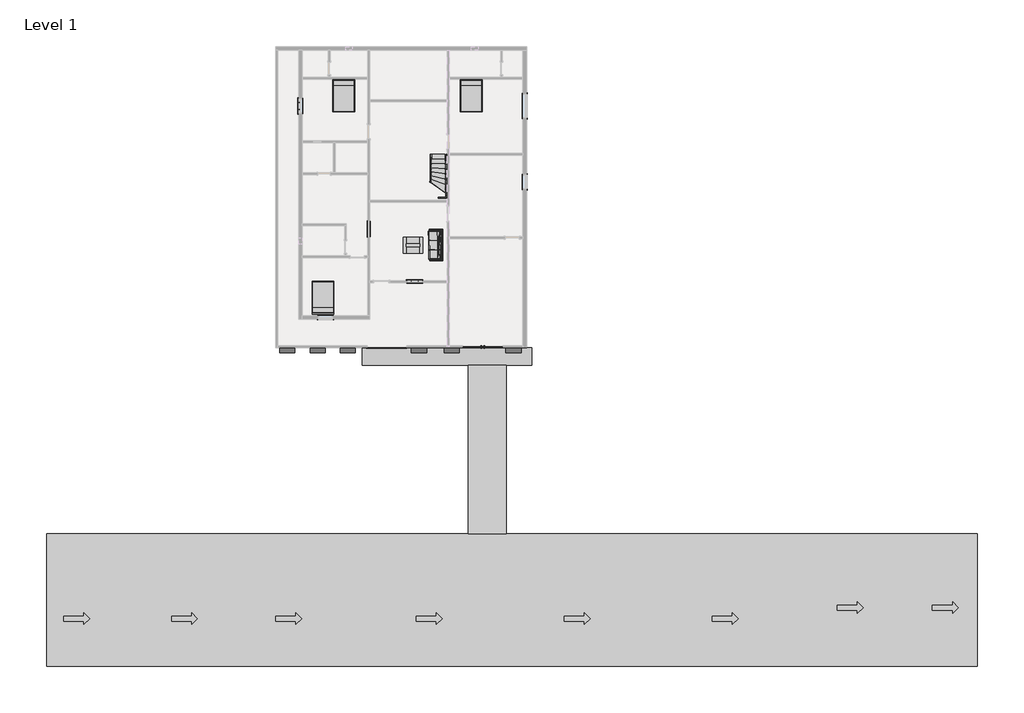
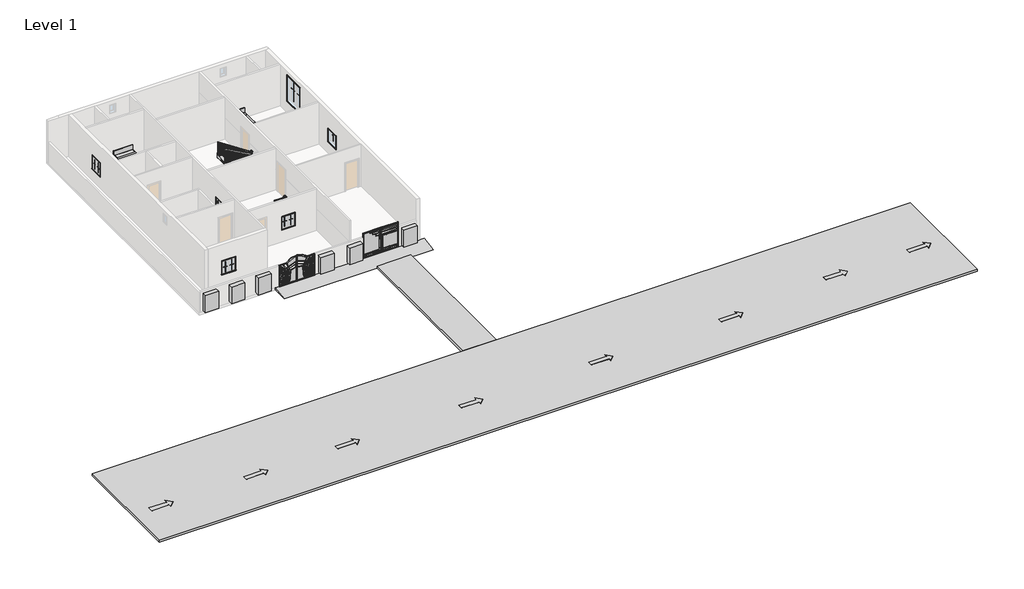
# One storey, part 3 of 3: 31 proxies, 8 geographic elements, 6 members, 5 furniture elements, 1 railing, 1 stair flight.
"""IFC4 building model written with IfcOpenShell, lengths in millimetres."""

from ifc_helpers import new_model, si_unit, frame, origin, place, context, project, spatial, polyline, outline, extrude, faceted_brep, transform, mapped, element, save
from components import generic_models_6bc30956, generic_models_113f6068, generic_models_1_generic_models_1_0d6a6266, generic_models_2_generic_models_2_5a51ac4f, generic_models_7_generic_models_7_b80b7fbc, generic_models_8_generic_models_8_37e38eb9, generic_models_9_generic_models_9_2e7d35d1, muntin_pattern_2x2_muntin_pattern_2x2_b3fe6957, muntin_pattern_2x2_muntin_pattern_2x2_3e0ecaf2, muntin_pattern_2x2_muntin_pattern_2x2_bff912c5, muntin_pattern_2x2_muntin_pattern_2x2_c2194282, trim_window_exterior_flat_with_sill_41619996, trim_window_exterior_flat_with_sill_e04b3088, trim_window_interior_flat_picture_frame_51c85655, trim_window_interior_flat_picture_frame_2a7685fe, furniture_2fc85b74, furniture_29a9adb8, furniture_57072a26, bed_17739_bed_17739_15c61121, wood_and_glass_coffee_table_17065_wood_and_glass_coffee_dbc724b2, direction_arrows_straight_direction_arrow_straight_a0d3235c, stair_flight_07df138c

model = new_model("IFC4")

# Units and contexts
model_context = context("Model", 3, world=origin())
ifc_project = project(units=[si_unit("LENGTHUNIT", "METRE", prefix="MILLI")], contexts=[model_context])

# Site, building, storey
site = spatial("IfcSite", under=ifc_project)
building = spatial("IfcBuilding", under=site)
storey = spatial("IfcBuildingStorey", under=building, Name="Level 1", Elevation=0.0)

# Proxies
placement = place(None, origin())
generic_models_shape = generic_models_6bc30956(model_context)
element("IfcBuildingElementProxy", 1, Name="Generic Models", at=placement, inside=storey, context=model_context, shape_type="MappedRepresentation", body=[
    mapped(generic_models_shape, transform((-2151.1799597, -7860.0977377, 0.0), x_axis=(1.0, 0.0, 0.0), y_axis=(0.0, 1.0, 0.0), z_axis=(0.0, 0.0, 1.0))),
])
generic_models_2_shape = generic_models_113f6068(model_context)
element("IfcBuildingElementProxy", 2, Name="Generic Models", at=placement, inside=storey, context=model_context, shape_type="MappedRepresentation", body=[
    mapped(generic_models_2_shape, transform((3685.0584916, -7809.2977377, 0.0), x_axis=(1.0, 0.0, 0.0), y_axis=(0.0, 1.0, 0.0), z_axis=(0.0, 0.0, 1.0))),
])
generic_models_1_generic_models_1_shape = generic_models_1_generic_models_1_0d6a6266(model_context)
element("IfcBuildingElementProxy", 3, Name="Generic Models 1 : Generic Models 1", ObjectType="Generic Models 1 : Generic Models 1", at=placement, inside=storey, context=model_context, shape_type="MappedRepresentation", body=[
    mapped(generic_models_1_generic_models_1_shape, transform((0.0, 0.0, 0.0), x_axis=(1.0, 0.0, 0.0), y_axis=(0.0, 1.0, 0.0), z_axis=(0.0, 0.0, 1.0))),
])
generic_models_2_generic_models_2_shape = generic_models_2_generic_models_2_5a51ac4f(model_context)
element("IfcBuildingElementProxy", 4, Name="Generic Models 2 : Generic Models 2", ObjectType="Generic Models 2 : Generic Models 2", at=placement, inside=storey, context=model_context, shape_type="MappedRepresentation", body=[
    mapped(generic_models_2_generic_models_2_shape, transform((0.0, 0.0, 0.0), x_axis=(1.0, 0.0, 0.0), y_axis=(0.0, 1.0, 0.0), z_axis=(0.0, 0.0, 1.0))),
])
generic_models_7_generic_models_7_shape = generic_models_7_generic_models_7_b80b7fbc(model_context)
element("IfcBuildingElementProxy", 5, Name="Generic Models 7 : Generic Models 7", ObjectType="Generic Models 7 : Generic Models 7", at=placement, inside=storey, context=model_context, shape_type="MappedRepresentation", body=[
    mapped(generic_models_7_generic_models_7_shape, transform((0.0, 0.0, 0.0), x_axis=(1.0, 0.0, 0.0), y_axis=(0.0, 1.0, 0.0), z_axis=(0.0, 0.0, 1.0))),
])
generic_models_8_generic_models_8_shape = generic_models_8_generic_models_8_37e38eb9(model_context)
element("IfcBuildingElementProxy", 6, Name="Generic Models 8 : Generic Models 8", ObjectType="Generic Models 8 : Generic Models 8", at=placement, inside=storey, context=model_context, shape_type="MappedRepresentation", body=[
    mapped(generic_models_8_generic_models_8_shape, transform((0.0, 0.0, 0.0), x_axis=(1.0, 0.0, 0.0), y_axis=(0.0, 1.0, 0.0), z_axis=(0.0, 0.0, 1.0))),
])
generic_models_9_generic_models_9_shape = generic_models_9_generic_models_9_2e7d35d1(model_context)
element("IfcBuildingElementProxy", 7, Name="Generic Models 9 : Generic Models 9", ObjectType="Generic Models 9 : Generic Models 9", at=placement, inside=storey, context=model_context, shape_type="MappedRepresentation", body=[
    mapped(generic_models_9_generic_models_9_shape, transform((0.0, -38.1, 0.0), x_axis=(1.0, 0.0, 0.0), y_axis=(0.0, 1.0, 0.0), z_axis=(0.0, 0.0, 1.0))),
])
muntin_pattern_2x2_muntin_pattern_2x2_shape = muntin_pattern_2x2_muntin_pattern_2x2_b3fe6957(model_context)
element("IfcBuildingElementProxy", 8, Name="Muntin Pattern_2x2 : Muntin Pattern_2x2", ObjectType="Muntin Pattern_2x2 : Muntin Pattern_2x2", at=placement, inside=storey, context=model_context, shape_type="MappedRepresentation", body=[
    mapped(muntin_pattern_2x2_muntin_pattern_2x2_shape, transform((-7494.1165084, 6600.4397623, 984.25), x_axis=(0.0, 1.0, 0.0), y_axis=(-1.0, 0.0, 0.0), z_axis=(0.0, 0.0, 1.0))),
])
element("IfcBuildingElementProxy", 9, Name="Muntin Pattern_2x2 : Muntin Pattern_2x2", ObjectType="Muntin Pattern_2x2 : Muntin Pattern_2x2", at=placement, inside=storey, context=model_context, shape_type="MappedRepresentation", body=[
    mapped(muntin_pattern_2x2_muntin_pattern_2x2_shape, transform((-5651.0290084, -6136.0727377, 984.25), x_axis=(-1.0, 0.0, 0.0), y_axis=(0.0, -1.0, 0.0), z_axis=(0.0, 0.0, 1.0))),
])
element("IfcBuildingElementProxy", 10, Name="Muntin Pattern_2x2 : Muntin Pattern_2x2", ObjectType="Muntin Pattern_2x2 : Muntin Pattern_2x2", at=placement, inside=storey, context=model_context, shape_type="MappedRepresentation", body=[
    mapped(muntin_pattern_2x2_muntin_pattern_2x2_shape, transform((-656.7540084, -3805.6227377, 984.25), x_axis=(1.0, 0.0, 0.0), y_axis=(0.0, 1.0, 0.0), z_axis=(0.0, 0.0, 1.0))),
])
element("IfcBuildingElementProxy", 11, Name="Muntin Pattern_2x2 : Muntin Pattern_2x2", ObjectType="Muntin Pattern_2x2 : Muntin Pattern_2x2", at=placement, inside=storey, context=model_context, shape_type="MappedRepresentation", body=[
    mapped(muntin_pattern_2x2_muntin_pattern_2x2_shape, transform((6355.2334916, 2418.9647623, 984.25), x_axis=(0.0, -1.0, 0.0), y_axis=(1.0, 0.0, 0.0), z_axis=(0.0, 0.0, 1.0))),
])
element("IfcBuildingElementProxy", 12, Name="Muntin Pattern_2x2 : Muntin Pattern_2x2", ObjectType="Muntin Pattern_2x2 : Muntin Pattern_2x2", at=placement, inside=storey, context=model_context, shape_type="MappedRepresentation", body=[
    mapped(muntin_pattern_2x2_muntin_pattern_2x2_shape, transform((-3277.7165084, -873.5102377, 984.25), x_axis=(0.0, 1.0, 0.0), y_axis=(-1.0, 0.0, 0.0), z_axis=(0.0, 0.0, 1.0))),
])
muntin_pattern_2x2_muntin_pattern_2x2_2_shape = muntin_pattern_2x2_muntin_pattern_2x2_3e0ecaf2(model_context)
element("IfcBuildingElementProxy", 13, Name="Muntin Pattern_2x2 : Muntin Pattern_2x2", ObjectType="Muntin Pattern_2x2 : Muntin Pattern_2x2", at=placement, inside=storey, context=model_context, shape_type="MappedRepresentation", body=[
    mapped(muntin_pattern_2x2_muntin_pattern_2x2_2_shape, transform((-7494.1165084, 7029.0647623, 984.25), x_axis=(0.0, -1.0, 0.0), y_axis=(1.0, 0.0, 0.0), z_axis=(0.0, 0.0, 1.0))),
])
element("IfcBuildingElementProxy", 14, Name="Muntin Pattern_2x2 : Muntin Pattern_2x2", ObjectType="Muntin Pattern_2x2 : Muntin Pattern_2x2", at=placement, inside=storey, context=model_context, shape_type="MappedRepresentation", body=[
    mapped(muntin_pattern_2x2_muntin_pattern_2x2_2_shape, transform((-6079.6540084, -6136.0727377, 984.25), x_axis=(1.0, 0.0, 0.0), y_axis=(0.0, 1.0, 0.0), z_axis=(0.0, 0.0, 1.0))),
])
element("IfcBuildingElementProxy", 15, Name="Muntin Pattern_2x2 : Muntin Pattern_2x2", ObjectType="Muntin Pattern_2x2 : Muntin Pattern_2x2", at=placement, inside=storey, context=model_context, shape_type="MappedRepresentation", body=[
    mapped(muntin_pattern_2x2_muntin_pattern_2x2_2_shape, transform((-228.1290084, -3805.6227377, 984.25), x_axis=(-1.0, 0.0, 0.0), y_axis=(0.0, -1.0, 0.0), z_axis=(0.0, 0.0, 1.0))),
])
element("IfcBuildingElementProxy", 16, Name="Muntin Pattern_2x2 : Muntin Pattern_2x2", ObjectType="Muntin Pattern_2x2 : Muntin Pattern_2x2", at=placement, inside=storey, context=model_context, shape_type="MappedRepresentation", body=[
    mapped(muntin_pattern_2x2_muntin_pattern_2x2_2_shape, transform((6355.2334916, 1990.3397623, 984.25), x_axis=(0.0, 1.0, 0.0), y_axis=(-1.0, 0.0, 0.0), z_axis=(0.0, 0.0, 1.0))),
])
element("IfcBuildingElementProxy", 17, Name="Muntin Pattern_2x2 : Muntin Pattern_2x2", ObjectType="Muntin Pattern_2x2 : Muntin Pattern_2x2", at=placement, inside=storey, context=model_context, shape_type="MappedRepresentation", body=[
    mapped(muntin_pattern_2x2_muntin_pattern_2x2_2_shape, transform((-3277.7165084, -444.8852377, 984.25), x_axis=(0.0, -1.0, 0.0), y_axis=(1.0, 0.0, 0.0), z_axis=(0.0, 0.0, 1.0))),
])
muntin_pattern_2x2_muntin_pattern_2x2_3_shape = muntin_pattern_2x2_muntin_pattern_2x2_bff912c5(model_context)
element("IfcBuildingElementProxy", 18, Name="Muntin Pattern_2x2 : Muntin Pattern_2x2", ObjectType="Muntin Pattern_2x2 : Muntin Pattern_2x2", at=placement, inside=storey, context=model_context, shape_type="MappedRepresentation", body=[
    mapped(muntin_pattern_2x2_muntin_pattern_2x2_3_shape, transform((6355.2334916, 7175.1147623, 984.25), x_axis=(0.0, -1.0, 0.0), y_axis=(1.0, 0.0, 0.0), z_axis=(0.0, 0.0, 1.0))),
])
muntin_pattern_2x2_muntin_pattern_2x2_4_shape = muntin_pattern_2x2_muntin_pattern_2x2_c2194282(model_context)
element("IfcBuildingElementProxy", 19, Name="Muntin Pattern_2x2 : Muntin Pattern_2x2", ObjectType="Muntin Pattern_2x2 : Muntin Pattern_2x2", at=placement, inside=storey, context=model_context, shape_type="MappedRepresentation", body=[
    mapped(muntin_pattern_2x2_muntin_pattern_2x2_4_shape, transform((6355.2334916, 6454.3897623, 984.25), x_axis=(0.0, 1.0, 0.0), y_axis=(-1.0, 0.0, 0.0), z_axis=(0.0, 0.0, 1.0))),
])
trim_window_exterior_flat_with_sill_shape = trim_window_exterior_flat_with_sill_41619996(model_context)
element("IfcBuildingElementProxy", 20, Name="Trim-Window-Exterior-Flat : with Sill", ObjectType="Trim-Window-Exterior-Flat : with Sill", at=placement, inside=storey, context=model_context, shape_type="MappedRepresentation", body=[
    mapped(trim_window_exterior_flat_with_sill_shape, transform((-7503.6415084, 6814.7522623, 1828.8), x_axis=(0.0, -1.0, 0.0), y_axis=(0.0, 0.0, 1.0), z_axis=(-1.0, 0.0, 0.0))),
])
element("IfcBuildingElementProxy", 21, Name="Trim-Window-Exterior-Flat : with Sill", ObjectType="Trim-Window-Exterior-Flat : with Sill", at=placement, inside=storey, context=model_context, shape_type="MappedRepresentation", body=[
    mapped(trim_window_exterior_flat_with_sill_shape, transform((-5865.3415084, -6145.5977377, 1828.8), x_axis=(1.0, 0.0, 0.0), y_axis=(0.0, 0.0, 1.0), z_axis=(0.0, -1.0, 0.0))),
])
element("IfcBuildingElementProxy", 22, Name="Trim-Window-Exterior-Flat : with Sill", ObjectType="Trim-Window-Exterior-Flat : with Sill", at=placement, inside=storey, context=model_context, shape_type="MappedRepresentation", body=[
    mapped(trim_window_exterior_flat_with_sill_shape, transform((-442.4415084, -3796.0977377, 1828.8), x_axis=(-1.0, 0.0, 0.0), y_axis=(0.0, 0.0, 1.0), z_axis=(0.0, 1.0, 0.0))),
])
element("IfcBuildingElementProxy", 23, Name="Trim-Window-Exterior-Flat : with Sill", ObjectType="Trim-Window-Exterior-Flat : with Sill", at=placement, inside=storey, context=model_context, shape_type="MappedRepresentation", body=[
    mapped(trim_window_exterior_flat_with_sill_shape, transform((6364.7584916, 2204.6522623, 1828.8), x_axis=(0.0, 1.0, 0.0), y_axis=(0.0, 0.0, 1.0), z_axis=(1.0, 0.0, 0.0))),
])
element("IfcBuildingElementProxy", 24, Name="Trim-Window-Exterior-Flat : with Sill", ObjectType="Trim-Window-Exterior-Flat : with Sill", at=placement, inside=storey, context=model_context, shape_type="MappedRepresentation", body=[
    mapped(trim_window_exterior_flat_with_sill_shape, transform((-3287.2415084, -659.1977377, 1828.8), x_axis=(0.0, -1.0, 0.0), y_axis=(0.0, 0.0, 1.0), z_axis=(-1.0, 0.0, 0.0))),
])
trim_window_exterior_flat_with_sill_2_shape = trim_window_exterior_flat_with_sill_e04b3088(model_context)
element("IfcBuildingElementProxy", 25, Name="Trim-Window-Exterior-Flat : with Sill", ObjectType="Trim-Window-Exterior-Flat : with Sill", at=placement, inside=storey, context=model_context, shape_type="MappedRepresentation", body=[
    mapped(trim_window_exterior_flat_with_sill_2_shape, transform((6364.7584916, 6814.7522623, 2743.2), x_axis=(0.0, 1.0, 0.0), y_axis=(0.0, 0.0, 1.0), z_axis=(1.0, 0.0, 0.0))),
])
trim_window_interior_flat_picture_frame_shape = trim_window_interior_flat_picture_frame_51c85655(model_context)
element("IfcBuildingElementProxy", 26, Name="Trim-Window-Interior-Flat : Picture Frame", ObjectType="Trim-Window-Interior-Flat : Picture Frame", at=placement, inside=storey, context=model_context, shape_type="MappedRepresentation", body=[
    mapped(trim_window_interior_flat_picture_frame_shape, transform((-7275.0415084, 6814.7522623, 1828.8), x_axis=(0.0, 1.0, 0.0), y_axis=(0.0, 0.0, 1.0), z_axis=(1.0, 0.0, 0.0))),
])
element("IfcBuildingElementProxy", 27, Name="Trim-Window-Interior-Flat : Picture Frame", ObjectType="Trim-Window-Interior-Flat : Picture Frame", at=placement, inside=storey, context=model_context, shape_type="MappedRepresentation", body=[
    mapped(trim_window_interior_flat_picture_frame_shape, transform((-5865.3415084, -5916.9977377, 1828.8), x_axis=(-1.0, 0.0, 0.0), y_axis=(0.0, 0.0, 1.0), z_axis=(0.0, 1.0, 0.0))),
])
element("IfcBuildingElementProxy", 28, Name="Trim-Window-Interior-Flat : Picture Frame", ObjectType="Trim-Window-Interior-Flat : Picture Frame", at=placement, inside=storey, context=model_context, shape_type="MappedRepresentation", body=[
    mapped(trim_window_interior_flat_picture_frame_shape, transform((-442.4415084, -3910.3977377, 1828.8), x_axis=(1.0, 0.0, 0.0), y_axis=(0.0, 0.0, 1.0), z_axis=(0.0, -1.0, 0.0))),
])
element("IfcBuildingElementProxy", 29, Name="Trim-Window-Interior-Flat : Picture Frame", ObjectType="Trim-Window-Interior-Flat : Picture Frame", at=placement, inside=storey, context=model_context, shape_type="MappedRepresentation", body=[
    mapped(trim_window_interior_flat_picture_frame_shape, transform((6136.1584916, 2204.6522623, 1828.8), x_axis=(0.0, -1.0, 0.0), y_axis=(0.0, 0.0, 1.0), z_axis=(-1.0, 0.0, 0.0))),
])
element("IfcBuildingElementProxy", 30, Name="Trim-Window-Interior-Flat : Picture Frame", ObjectType="Trim-Window-Interior-Flat : Picture Frame", at=placement, inside=storey, context=model_context, shape_type="MappedRepresentation", body=[
    mapped(trim_window_interior_flat_picture_frame_shape, transform((-3172.9415084, -659.1977377, 1828.8), x_axis=(0.0, 1.0, 0.0), y_axis=(0.0, 0.0, 1.0), z_axis=(1.0, 0.0, 0.0))),
])
trim_window_interior_flat_picture_frame_2_shape = trim_window_interior_flat_picture_frame_2a7685fe(model_context)
element("IfcBuildingElementProxy", 31, Name="Trim-Window-Interior-Flat : Picture Frame", ObjectType="Trim-Window-Interior-Flat : Picture Frame", at=placement, inside=storey, context=model_context, shape_type="MappedRepresentation", body=[
    mapped(trim_window_interior_flat_picture_frame_2_shape, transform((6136.1584916, 6814.7522623, 2743.2), x_axis=(0.0, -1.0, 0.0), y_axis=(0.0, 0.0, 1.0), z_axis=(-1.0, 0.0, 0.0))),
])

# Furniture
furniture_shape = furniture_2fc85b74(model_context)
furniture_2_shape = furniture_29a9adb8(model_context)
furniture_3_shape = furniture_57072a26(model_context)
element("IfcFurniture", 32, at=placement, inside=storey, context=model_context, shape_type="MappedRepresentation", body=[
    mapped(furniture_shape, transform((460.7695276, -1640.1238257, 0.0), x_axis=(0.014042050983927294, -0.9999014055416489, 0.0), y_axis=(0.9999014055416489, 0.014042050983927294, 0.0), z_axis=(0.0, 0.0, 1.0))),
    mapped(furniture_2_shape, transform((460.7695276, -1640.1238257, 0.0), x_axis=(0.014042050983927294, -0.9999014055416489, 0.0), y_axis=(0.9999014055416489, 0.014042050983927294, 0.0), z_axis=(0.0, 0.0, 1.0))),
    mapped(furniture_3_shape, transform((460.7695276, -1640.1238257, 0.0), x_axis=(0.014042050983927294, -0.9999014055416489, 0.0), y_axis=(0.9999014055416489, 0.014042050983927294, 0.0), z_axis=(0.0, 0.0, 1.0))),
])
bed_17739_bed_17739_shape = bed_17739_bed_17739_15c61121(model_context)
element("IfcFurniture", 33, ObjectType="Bed_17739 : Bed_17739", at=placement, inside=storey, context=model_context, shape_type="MappedRepresentation", body=[
    mapped(bed_17739_bed_17739_shape, transform((-4754.0915084, 7424.3522623, 0.0), x_axis=(1.0, 0.0, 0.0), y_axis=(0.0, 1.0, 0.0), z_axis=(0.0, 0.0, 1.0))),
])
element("IfcFurniture", 34, ObjectType="Bed_17739 : Bed_17739", at=placement, inside=storey, context=model_context, shape_type="MappedRepresentation", body=[
    mapped(bed_17739_bed_17739_shape, transform((2998.5366507, 7424.3522623, 0.0), x_axis=(1.0, 0.0, 0.0), y_axis=(0.0, 1.0, 0.0), z_axis=(0.0, 0.0, 1.0))),
])
element("IfcFurniture", 35, ObjectType="Bed_17739 : Bed_17739", at=placement, inside=storey, context=model_context, shape_type="MappedRepresentation", body=[
    mapped(bed_17739_bed_17739_shape, transform((-6017.7415084, -4812.0977377, 0.0), x_axis=(-1.0, 0.0, 0.0), y_axis=(0.0, -1.0, 0.0), z_axis=(0.0, 0.0, 1.0))),
])
wood_and_glass_coffee_table_17065_wood_and_glass_coffee_shape = wood_and_glass_coffee_table_17065_wood_and_glass_coffee_dbc724b2(model_context)
element("IfcFurniture", 36, ObjectType="Wood_and_Glass_Coffee_Table_17065 : Wood_and_Glass_Coffee_Table_17065", at=placement, inside=storey, context=model_context, shape_type="MappedRepresentation", body=[
    mapped(wood_and_glass_coffee_table_17065_wood_and_glass_coffee_shape, transform((-550.3915084, -1643.4477377, 0.0), x_axis=(1.0, 0.0, 0.0), y_axis=(0.0, 1.0, 0.0), z_axis=(0.0, 0.0, 1.0))),
])

# Geographic elements
direction_arrows_straight_direction_arrow_straight_shape = direction_arrows_straight_direction_arrow_straight_a0d3235c(model_context)
element("IfcGeographicElement", 37, ObjectType="Direction Arrows - Straight : Direction Arrow - Straight", at=placement, inside=storey, context=model_context, shape_type="MappedRepresentation", body=[
    mapped(direction_arrows_straight_direction_arrow_straight_shape, transform((-15218.8915084, -24331.9977377, 152.4), x_axis=(0.0, -1.0, 0.0), y_axis=(1.0, 0.0, 0.0), z_axis=(0.0, 0.0, 1.0))),
])
element("IfcGeographicElement", 38, ObjectType="Direction Arrows - Straight : Direction Arrow - Straight", at=placement, inside=storey, context=model_context, shape_type="MappedRepresentation", body=[
    mapped(direction_arrows_straight_direction_arrow_straight_shape, transform((-21772.0915084, -24331.9977377, 152.4), x_axis=(0.0, -1.0, 0.0), y_axis=(1.0, 0.0, 0.0), z_axis=(0.0, 0.0, 1.0))),
])
element("IfcGeographicElement", 39, ObjectType="Direction Arrows - Straight : Direction Arrow - Straight", at=placement, inside=storey, context=model_context, shape_type="MappedRepresentation", body=[
    mapped(direction_arrows_straight_direction_arrow_straight_shape, transform((-8881.8069473, -24331.9977377, 152.4), x_axis=(0.0, -1.0, 0.0), y_axis=(1.0, 0.0, 0.0), z_axis=(0.0, 0.0, 1.0))),
])
element("IfcGeographicElement", 40, ObjectType="Direction Arrows - Straight : Direction Arrow - Straight", at=placement, inside=storey, context=model_context, shape_type="MappedRepresentation", body=[
    mapped(direction_arrows_straight_direction_arrow_straight_shape, transform((-347.4069473, -24331.9977377, 152.4), x_axis=(0.0, -1.0, 0.0), y_axis=(1.0, 0.0, 0.0), z_axis=(0.0, 0.0, 1.0))),
])
element("IfcGeographicElement", 41, ObjectType="Direction Arrows - Straight : Direction Arrow - Straight", at=placement, inside=storey, context=model_context, shape_type="MappedRepresentation", body=[
    mapped(direction_arrows_straight_direction_arrow_straight_shape, transform((8644.1930527, -24331.9977377, 152.4), x_axis=(0.0, -1.0, 0.0), y_axis=(1.0, 0.0, 0.0), z_axis=(0.0, 0.0, 1.0))),
])
element("IfcGeographicElement", 42, ObjectType="Direction Arrows - Straight : Direction Arrow - Straight", at=placement, inside=storey, context=model_context, shape_type="MappedRepresentation", body=[
    mapped(direction_arrows_straight_direction_arrow_straight_shape, transform((17635.7930527, -24331.9977377, 152.4), x_axis=(0.0, -1.0, 0.0), y_axis=(1.0, 0.0, 0.0), z_axis=(0.0, 0.0, 1.0))),
])
element("IfcGeographicElement", 43, ObjectType="Direction Arrows - Straight : Direction Arrow - Straight", at=placement, inside=storey, context=model_context, shape_type="MappedRepresentation", body=[
    mapped(direction_arrows_straight_direction_arrow_straight_shape, transform((25226.7966521, -23667.870978, 152.4), x_axis=(0.0, -1.0, 0.0), y_axis=(1.0, 0.0, 0.0), z_axis=(0.0, 0.0, 1.0))),
])
element("IfcGeographicElement", 44, ObjectType="Direction Arrows - Straight : Direction Arrow - Straight", at=placement, inside=storey, context=model_context, shape_type="MappedRepresentation", body=[
    mapped(direction_arrows_straight_direction_arrow_straight_shape, transform((31017.9966521, -23667.870978, 152.4), x_axis=(0.0, -1.0, 0.0), y_axis=(1.0, 0.0, 0.0), z_axis=(0.0, 0.0, 1.0))),
])

# Members
element("IfcMember", 45, ObjectType="Stringer - 2\" Width", at=placement, inside=storey, context=model_context, shape_type="SweptSolid", body=[
    extrude(outline(polyline([(3870.4222402, 233.6789033), (3870.4222402, 0.0), (3655.4968958, 0.0), (1369.1992084, 1132.6067011), (1369.1992084, 1472.7572536), (3870.4222402, 233.6789033)])), frame((1456.2084916, 0.0, 0.0), z_axis=(1.0, 0.0, 0.0), x_axis=(0.0, 1.0, 0.0)), (0.0, 0.0, 1.0), 50.8),
])
element("IfcMember", 46, ObjectType="Stringer - 2\" Width", at=placement, inside=storey, context=model_context, shape_type="SweptSolid", body=[
    extrude(outline(polyline([(1456.2084916, 1369.1992084), (1507.0084916, 1369.1992084), (1507.0084916, 1218.1652728), (1456.2084916, 1268.9652728), (1456.2084916, 1369.1992084)])), frame((0.0, 0.0, 1132.6067011), z_axis=(0.0, 0.0, 1.0), x_axis=(1.0, 0.0, 0.0)), (0.0, 0.0, 1.0), 340.1505525),
])
element("IfcMember", 47, ObjectType="Stringer - 2\" Width", at=placement, inside=storey, context=model_context, shape_type="SweptSolid", body=[
    extrude(outline(polyline([(1456.2084916, 1268.9652728), (1507.0084916, 1218.1652728), (1113.208453, 1218.1652728), (1113.208453, 1268.9652728), (1456.2084916, 1268.9652728)])), frame((0.0, 0.0, 1132.6067011), z_axis=(0.0, 0.0, 1.0), x_axis=(1.0, 0.0, 0.0)), (0.0, 0.0, 1.0), 340.1505525),
])
element("IfcMember", 48, ObjectType="Stringer - 2\" Width", at=placement, inside=storey, context=model_context, shape_type="SweptSolid", body=[
    extrude(outline(polyline([(3870.4222402, 190.2545013), (3870.4222402, 0.0), (3614.0281198, 0.0), (2234.1652728, 1006.4313584), (2234.1652728, 1383.6921868), (3870.4222402, 190.2545013)])), frame((491.0084916, 0.0, 0.0), z_axis=(1.0, 0.0, 0.0), x_axis=(0.0, 1.0, 0.0)), (0.0, 0.0, 1.0), 50.8),
])
element("IfcMember", 49, ObjectType="Stringer - 2\" Width", at=placement, inside=storey, context=model_context, shape_type="SweptSolid", body=[
    extrude(outline(polyline([(1158.1835681, 541.8084916), (1525.9965617, 541.8084916), (3116.9897736, -1813.7050583), (2749.17678, -1813.7050583), (1158.1835681, 541.8084916)])), frame((0.0, 2183.3652728, 0.0), z_axis=(0.0, 1.0, 0.0), x_axis=(0.0, 0.0, 1.0)), (0.0, 0.0, 1.0), 50.8),
])
element("IfcMember", 50, ObjectType="Stringer - 2\" Width", at=placement, inside=storey, context=model_context, shape_type="SweptSolid", body=[
    extrude(outline(polyline([(1132.6067011, 1113.208453), (1472.7572536, 1113.208453), (3063.9877281, -1813.7050583), (2723.8371756, -1813.7050583), (1132.6067011, 1113.208453)])), frame((0.0, 1218.1652728, 0.0), z_axis=(0.0, 1.0, 0.0), x_axis=(0.0, 0.0, 1.0)), (0.0, 0.0, 1.0), 50.8),
])

# Railing
element("IfcRailing", 51, ObjectType="Handrail - Rectangular", at=placement, inside=storey, context=model_context, shape_type="SolidModel", body=[
    faceted_brep([(592.6084916, 3870.4222402, 1083.7333333), (592.6084916, 3870.4222402, 1021.4674881), (541.8084916, 3870.4222402, 1021.4674881), (541.8084916, 3870.4222402, 1083.7333333), (592.6084916, 2259.5652728, 2225.4596781), (592.6084916, 2208.7652728, 2199.1993253), (541.8084916, 2208.7652728, 2199.1993253), (541.8084916, 2259.5652728, 2225.4596781), (592.6084916, 2259.5652728, 2442.2092282), (592.6084916, 2208.7652728, 2391.4092282), (541.8084916, 2208.7652728, 2391.4092282), (541.8084916, 2259.5652728, 2442.2092282), (592.6084916, 2132.5652728, 2442.2092282), (592.6084916, 2132.5652728, 2391.4092282), (541.8084916, 2183.3652728, 2391.4092282), (541.8084916, 2183.3652728, 2442.2092282), (465.6084916, 2132.5652728, 2442.2092282), (450.2220288, 2132.5652728, 2391.4092282), (450.2220288, 2183.3652728, 2391.4092282), (465.6084916, 2183.3652728, 2442.2092282), (-1813.7050583, 2132.5652728, 3962.4), (-1813.7050583, 2183.3652728, 3962.4), (-1813.7050583, 2183.3652728, 3901.3379811), (-1813.7050583, 2132.5652728, 3901.3379811)], [[[0, 1, 2, 3]], [[1, 0, 4, 5]], [[2, 1, 5, 6]], [[3, 2, 6, 7]], [[0, 3, 7, 4]], [[5, 4, 8, 9]], [[6, 5, 9, 10]], [[7, 6, 10, 11]], [[4, 7, 11, 8]], [[9, 8, 12, 13]], [[10, 9, 13, 14]], [[11, 10, 14, 15]], [[8, 11, 15, 12]], [[13, 12, 16, 17]], [[14, 13, 17, 18]], [[15, 14, 18, 19]], [[12, 15, 19, 16]], [[20, 21, 22, 23]], [[17, 16, 20, 23]], [[18, 17, 23, 22]], [[19, 18, 22, 21]], [[16, 19, 21, 20]]]),
    extrude(outline(polyline([(3865.5636891, -1760.0665084), (3878.2691083, -1779.1165084), (2878.6666667, -1779.1165084), (2878.6666667, -1760.0665084), (3865.5636891, -1760.0665084)])), frame((0.0, 2148.4402728, 0.0), z_axis=(0.0, 1.0, 0.0), x_axis=(0.0, 0.0, 1.0)), (0.0, 0.0, 1.0), 19.05),
    extrude(outline(polyline([(3797.8014532, -1658.4665084), (3810.5068724, -1677.5165084), (2878.6666667, -1677.5165084), (2878.6666667, -1658.4665084), (3797.8014532, -1658.4665084)])), frame((0.0, 2148.4402728, 0.0), z_axis=(0.0, 1.0, 0.0), x_axis=(0.0, 0.0, 1.0)), (0.0, 0.0, 1.0), 19.05),
    extrude(outline(polyline([(3730.0392173, -1556.8665084), (3742.7446365, -1575.9165084), (2878.6666667, -1575.9165084), (2878.6666667, -1556.8665084), (3730.0392173, -1556.8665084)])), frame((0.0, 2148.4402728, 0.0), z_axis=(0.0, 1.0, 0.0), x_axis=(0.0, 0.0, 1.0)), (0.0, 0.0, 1.0), 19.05),
    extrude(outline(polyline([(3662.1324687, -1455.2665084), (3674.8378879, -1474.3165084), (2709.3333333, -1474.3165084), (2709.3333333, -1455.2665084), (3662.1324687, -1455.2665084)])), frame((0.0, 2148.4402728, 0.0), z_axis=(0.0, 1.0, 0.0), x_axis=(0.0, 0.0, 1.0)), (0.0, 0.0, 1.0), 19.05),
    extrude(outline(polyline([(3594.3702328, -1353.6665084), (3607.075652, -1372.7165084), (2709.3333333, -1372.7165084), (2709.3333333, -1353.6665084), (3594.3702328, -1353.6665084)])), frame((0.0, 2148.4402728, 0.0), z_axis=(0.0, 1.0, 0.0), x_axis=(0.0, 0.0, 1.0)), (0.0, 0.0, 1.0), 19.05),
    extrude(outline(polyline([(3526.6079969, -1252.0665084), (3539.3134161, -1271.1165084), (2709.3333333, -1271.1165084), (2709.3333333, -1252.0665084), (3526.6079969, -1252.0665084)])), frame((0.0, 2148.4402728, 0.0), z_axis=(0.0, 1.0, 0.0), x_axis=(0.0, 0.0, 1.0)), (0.0, 0.0, 1.0), 19.05),
    extrude(outline(polyline([(3459.1347865, -1150.4665084), (3471.8402057, -1169.5165084), (2540.0, -1169.5165084), (2540.0, -1150.4665084), (3459.1347865, -1150.4665084)])), frame((0.0, 2148.4402728, 0.0), z_axis=(0.0, 1.0, 0.0), x_axis=(0.0, 0.0, 1.0)), (0.0, 0.0, 1.0), 19.05),
    extrude(outline(polyline([(3391.3725506, -1048.8665084), (3404.0779698, -1067.9165084), (2540.0, -1067.9165084), (2540.0, -1048.8665084), (3391.3725506, -1048.8665084)])), frame((0.0, 2148.4402728, 0.0), z_axis=(0.0, 1.0, 0.0), x_axis=(0.0, 0.0, 1.0)), (0.0, 0.0, 1.0), 19.05),
    extrude(outline(polyline([(3323.465802, -947.2665084), (3336.1712212, -966.3165084), (2370.6666667, -966.3165084), (2370.6666667, -947.2665084), (3323.465802, -947.2665084)])), frame((0.0, 2148.4402728, 0.0), z_axis=(0.0, 1.0, 0.0), x_axis=(0.0, 0.0, 1.0)), (0.0, 0.0, 1.0), 19.05),
    extrude(outline(polyline([(3255.7035661, -845.6665084), (3268.4089853, -864.7165084), (2370.6666667, -864.7165084), (2370.6666667, -845.6665084), (3255.7035661, -845.6665084)])), frame((0.0, 2148.4402728, 0.0), z_axis=(0.0, 1.0, 0.0), x_axis=(0.0, 0.0, 1.0)), (0.0, 0.0, 1.0), 19.05),
    extrude(outline(polyline([(3187.9413302, -744.0665084), (3200.6467495, -763.1165084), (2370.6666667, -763.1165084), (2370.6666667, -744.0665084), (3187.9413302, -744.0665084)])), frame((0.0, 2148.4402728, 0.0), z_axis=(0.0, 1.0, 0.0), x_axis=(0.0, 0.0, 1.0)), (0.0, 0.0, 1.0), 19.05),
    extrude(outline(polyline([(3120.1790943, -642.4665084), (3132.8845136, -661.5165084), (2201.3333333, -661.5165084), (2201.3333333, -642.4665084), (3120.1790943, -642.4665084)])), frame((0.0, 2148.4402728, 0.0), z_axis=(0.0, 1.0, 0.0), x_axis=(0.0, 0.0, 1.0)), (0.0, 0.0, 1.0), 19.05),
    extrude(outline(polyline([(3052.4168585, -540.8665084), (3065.1222777, -559.9165084), (2201.3333333, -559.9165084), (2201.3333333, -540.8665084), (3052.4168585, -540.8665084)])), frame((0.0, 2148.4402728, 0.0), z_axis=(0.0, 1.0, 0.0), x_axis=(0.0, 0.0, 1.0)), (0.0, 0.0, 1.0), 19.05),
    extrude(outline(polyline([(2984.5101098, -439.2665084), (2997.2155291, -458.3165084), (2201.3333333, -458.3165084), (2201.3333333, -439.2665084), (2984.5101098, -439.2665084)])), frame((0.0, 2148.4402728, 0.0), z_axis=(0.0, 1.0, 0.0), x_axis=(0.0, 0.0, 1.0)), (0.0, 0.0, 1.0), 19.05),
    extrude(outline(polyline([(2917.0368994, -337.6665084), (2929.7423187, -356.7165084), (2032.0, -356.7165084), (2032.0, -337.6665084), (2917.0368994, -337.6665084)])), frame((0.0, 2148.4402728, 0.0), z_axis=(0.0, 1.0, 0.0), x_axis=(0.0, 0.0, 1.0)), (0.0, 0.0, 1.0), 19.05),
    extrude(outline(polyline([(2849.2746636, -236.0665084), (2861.9800828, -255.1165084), (2032.0, -255.1165084), (2032.0, -236.0665084), (2849.2746636, -236.0665084)])), frame((0.0, 2148.4402728, 0.0), z_axis=(0.0, 1.0, 0.0), x_axis=(0.0, 0.0, 1.0)), (0.0, 0.0, 1.0), 19.05),
    extrude(outline(polyline([(2781.5124277, -134.4665084), (2794.2178469, -153.5165084), (1862.6666667, -153.5165084), (1862.6666667, -134.4665084), (2781.5124277, -134.4665084)])), frame((0.0, 2148.4402728, 0.0), z_axis=(0.0, 1.0, 0.0), x_axis=(0.0, 0.0, 1.0)), (0.0, 0.0, 1.0), 19.05),
    extrude(outline(polyline([(2713.7501918, -32.8665084), (2726.455611, -51.9165084), (1862.6666667, -51.9165084), (1862.6666667, -32.8665084), (2713.7501918, -32.8665084)])), frame((0.0, 2148.4402728, 0.0), z_axis=(0.0, 1.0, 0.0), x_axis=(0.0, 0.0, 1.0)), (0.0, 0.0, 1.0), 19.05),
    extrude(outline(polyline([(2645.8434432, 68.7334916), (2658.5488624, 49.6834916), (1862.6666667, 49.6834916), (1862.6666667, 68.7334916), (2645.8434432, 68.7334916)])), frame((0.0, 2148.4402728, 0.0), z_axis=(0.0, 1.0, 0.0), x_axis=(0.0, 0.0, 1.0)), (0.0, 0.0, 1.0), 19.05),
    extrude(outline(polyline([(2578.0812073, 170.3334916), (2590.7866265, 151.2834916), (1693.3333333, 151.2834916), (1693.3333333, 170.3334916), (2578.0812073, 170.3334916)])), frame((0.0, 2148.4402728, 0.0), z_axis=(0.0, 1.0, 0.0), x_axis=(0.0, 0.0, 1.0)), (0.0, 0.0, 1.0), 19.05),
    extrude(outline(polyline([(2510.3189714, 271.9334916), (2523.0243906, 252.8834916), (1693.3333333, 252.8834916), (1693.3333333, 271.9334916), (2510.3189714, 271.9334916)])), frame((0.0, 2148.4402728, 0.0), z_axis=(0.0, 1.0, 0.0), x_axis=(0.0, 0.0, 1.0)), (0.0, 0.0, 1.0), 19.05),
    extrude(outline(polyline([(2442.5567355, 373.5334916), (2455.2621547, 354.4834916), (1524.0, 354.4834916), (1524.0, 373.5334916), (2442.5567355, 373.5334916)])), frame((0.0, 2148.4402728, 0.0), z_axis=(0.0, 1.0, 0.0), x_axis=(0.0, 0.0, 1.0)), (0.0, 0.0, 1.0), 19.05),
    extrude(outline(polyline([(2374.7944996, 475.1334916), (2387.4999189, 456.0834916), (1524.0, 456.0834916), (1524.0, 475.1334916), (2374.7944996, 475.1334916)])), frame((0.0, 2148.4402728, 0.0), z_axis=(0.0, 1.0, 0.0), x_axis=(0.0, 0.0, 1.0)), (0.0, 0.0, 1.0), 19.05),
    extrude(outline(polyline([(557.6834916, 2254.3472402), (576.7334916, 2254.3472402), (576.7334916, 2235.2972402), (557.6834916, 2235.2972402), (557.6834916, 2254.3472402)])), frame((0.0, 0.0, 1185.3333333), z_axis=(0.0, 0.0, 1.0), x_axis=(1.0, 0.0, 0.0)), (0.0, 0.0, 1.0), 1206.0758948),
    extrude(outline(polyline([(2336.8972402, 2108.3832902), (2355.9472402, 2094.8812306), (2355.9472402, 1185.3333333), (2336.8972402, 1185.3333333), (2336.8972402, 2108.3832902)])), frame((557.6834916, 0.0, 0.0), z_axis=(1.0, 0.0, 0.0), x_axis=(0.0, 1.0, 0.0)), (0.0, 0.0, 1.0), 19.05),
    extrude(outline(polyline([(2438.4972402, 2036.3723054), (2457.5472402, 2022.8702458), (2457.5472402, 1016.0), (2438.4972402, 1016.0), (2438.4972402, 2036.3723054)])), frame((557.6834916, 0.0, 0.0), z_axis=(1.0, 0.0, 0.0), x_axis=(0.0, 1.0, 0.0)), (0.0, 0.0, 1.0), 19.05),
    extrude(outline(polyline([(2540.0972402, 1964.3613206), (2559.1472402, 1950.8592609), (2559.1472402, 1016.0), (2540.0972402, 1016.0), (2540.0972402, 1964.3613206)])), frame((557.6834916, 0.0, 0.0), z_axis=(1.0, 0.0, 0.0), x_axis=(0.0, 1.0, 0.0)), (0.0, 0.0, 1.0), 19.05),
    extrude(outline(polyline([(2641.6972402, 1892.3503358), (2660.7472402, 1878.8482761), (2660.7472402, 846.6666667), (2641.6972402, 846.6666667), (2641.6972402, 1892.3503358)])), frame((557.6834916, 0.0, 0.0), z_axis=(1.0, 0.0, 0.0), x_axis=(0.0, 1.0, 0.0)), (0.0, 0.0, 1.0), 19.05),
    extrude(outline(polyline([(2743.2972402, 1820.339351), (2762.3472402, 1806.8372913), (2762.3472402, 846.6666667), (2743.2972402, 846.6666667), (2743.2972402, 1820.339351)])), frame((557.6834916, 0.0, 0.0), z_axis=(1.0, 0.0, 0.0), x_axis=(0.0, 1.0, 0.0)), (0.0, 0.0, 1.0), 19.05),
    extrude(outline(polyline([(2844.8972402, 1748.3283661), (2863.9472402, 1734.8263065), (2863.9472402, 677.3333333), (2844.8972402, 677.3333333), (2844.8972402, 1748.3283661)])), frame((557.6834916, 0.0, 0.0), z_axis=(1.0, 0.0, 0.0), x_axis=(0.0, 1.0, 0.0)), (0.0, 0.0, 1.0), 19.05),
    extrude(outline(polyline([(2946.4972402, 1676.3173813), (2965.5472402, 1662.8153217), (2965.5472402, 677.3333333), (2946.4972402, 677.3333333), (2946.4972402, 1676.3173813)])), frame((557.6834916, 0.0, 0.0), z_axis=(1.0, 0.0, 0.0), x_axis=(0.0, 1.0, 0.0)), (0.0, 0.0, 1.0), 19.05),
    extrude(outline(polyline([(3048.0972402, 1604.3063965), (3067.1472402, 1590.8043368), (3067.1472402, 508.0), (3048.0972402, 508.0), (3048.0972402, 1604.3063965)])), frame((557.6834916, 0.0, 0.0), z_axis=(1.0, 0.0, 0.0), x_axis=(0.0, 1.0, 0.0)), (0.0, 0.0, 1.0), 19.05),
    extrude(outline(polyline([(3149.6972402, 1532.2954117), (3168.7472402, 1518.793352), (3168.7472402, 508.0), (3149.6972402, 508.0), (3149.6972402, 1532.2954117)])), frame((557.6834916, 0.0, 0.0), z_axis=(1.0, 0.0, 0.0), x_axis=(0.0, 1.0, 0.0)), (0.0, 0.0, 1.0), 19.05),
    extrude(outline(polyline([(3251.2972402, 1460.2844268), (3270.3472402, 1446.7823672), (3270.3472402, 508.0), (3251.2972402, 508.0), (3251.2972402, 1460.2844268)])), frame((557.6834916, 0.0, 0.0), z_axis=(1.0, 0.0, 0.0), x_axis=(0.0, 1.0, 0.0)), (0.0, 0.0, 1.0), 19.05),
    extrude(outline(polyline([(3352.8972402, 1388.273442), (3371.9472402, 1374.7713824), (3371.9472402, 338.6666667), (3352.8972402, 338.6666667), (3352.8972402, 1388.273442)])), frame((557.6834916, 0.0, 0.0), z_axis=(1.0, 0.0, 0.0), x_axis=(0.0, 1.0, 0.0)), (0.0, 0.0, 1.0), 19.05),
    extrude(outline(polyline([(3454.4972402, 1316.2624572), (3473.5472402, 1302.7603976), (3473.5472402, 338.6666667), (3454.4972402, 338.6666667), (3454.4972402, 1316.2624572)])), frame((557.6834916, 0.0, 0.0), z_axis=(1.0, 0.0, 0.0), x_axis=(0.0, 1.0, 0.0)), (0.0, 0.0, 1.0), 19.05),
    extrude(outline(polyline([(3556.0972402, 1244.2514724), (3575.1472402, 1230.7494127), (3575.1472402, 338.6666667), (3556.0972402, 338.6666667), (3556.0972402, 1244.2514724)])), frame((557.6834916, 0.0, 0.0), z_axis=(1.0, 0.0, 0.0), x_axis=(0.0, 1.0, 0.0)), (0.0, 0.0, 1.0), 19.05),
    extrude(outline(polyline([(3657.6972402, 1172.2404876), (3676.7472402, 1158.7384279), (3676.7472402, 169.3333333), (3657.6972402, 169.3333333), (3657.6972402, 1172.2404876)])), frame((557.6834916, 0.0, 0.0), z_axis=(1.0, 0.0, 0.0), x_axis=(0.0, 1.0, 0.0)), (0.0, 0.0, 1.0), 19.05),
    extrude(outline(polyline([(3759.2972402, 1100.2295027), (3778.3472402, 1086.7274431), (3778.3472402, 169.3333333), (3759.2972402, 169.3333333), (3759.2972402, 1100.2295027)])), frame((557.6834916, 0.0, 0.0), z_axis=(1.0, 0.0, 0.0), x_axis=(0.0, 1.0, 0.0)), (0.0, 0.0, 1.0), 19.05),
    extrude(outline(polyline([(557.6834916, 2167.4902728), (576.7334916, 2167.4902728), (576.7334916, 2148.4402728), (557.6834916, 2148.4402728), (557.6834916, 2167.4902728)])), frame((0.0, 0.0, 1354.6666667), z_axis=(0.0, 0.0, 1.0), x_axis=(1.0, 0.0, 0.0)), (0.0, 0.0, 1.0), 1036.7425615),
    extrude(outline(polyline([(3888.6325619, -1794.6550583), (3901.3379811, -1813.7050583), (2878.6666667, -1813.7050583), (2878.6666667, -1794.6550583), (3888.6325619, -1794.6550583)])), frame((0.0, 2148.4402728, 0.0), z_axis=(0.0, 1.0, 0.0), x_axis=(0.0, 0.0, 1.0)), (0.0, 0.0, 1.0), 19.05),
    extrude(outline(polyline([(3851.3722402, 1034.9695477), (3870.4222402, 1021.4674881), (3870.4222402, 169.3333333), (3851.3722402, 169.3333333), (3851.3722402, 1034.9695477)])), frame((557.6834916, 0.0, 0.0), z_axis=(1.0, 0.0, 0.0), x_axis=(0.0, 1.0, 0.0)), (0.0, 0.0, 1.0), 19.05),
])

# Stair flight
stair_flight_shape = stair_flight_07df138c(model_context)
element("IfcStairFlight", 52, ObjectType="2\" Tread 1\" Nosing 1/4\" Riser", at=placement, inside=storey, context=model_context, shape_type="MappedRepresentation", body=[
    mapped(stair_flight_shape, transform((0.0, 0.0, 0.0), x_axis=(1.0, 0.0, 0.0), y_axis=(0.0, 1.0, 0.0), z_axis=(0.0, 0.0, 1.0))),
])

save(model, "model.ifc")

# Revit data of these elements
# Type
#   m.s. sheet = none
#   2" x2" pipe = none
#   1"x1"pipe = none
#   Default Elevation = 0
# Type
#   sheet = none
#   pipe = none
#   handal = none
#   faram = none
#   Default Elevation = 0
# Type "Muntin Pattern_2x2 : Muntin Pattern_2x2"
#   Width [instance default] = 4' - 0"
#   Thickness = 0' - 0 1/2"
#   Height [instance default] = 4' - 0"
#   Distance = 0' - 0 3/4"
#   Interior Material [instance default] = none
#   Exterior Material [instance default] = none
#   Default Elevation = 0
# Type "Trim-Window-Exterior-Flat : with Sill"
#   Trim Width = 0' - 2 1/4"
#   Trim Thickness_Picture Frame = 0' - 1 1/4"
#   Trim Thickness_with Sill = 0' - 0 3/4"
#   Sill Thickness = 0' - 1 1/4"
#   Opening Width [instance default] = 2' - 0"
#   Opening Height [instance default] = 3' - 0"
#   Default Elevation = 4' - 0"
#   Sill = yes
#   Picture Frame = no
#   Trim Material [instance default] = none
# Type "Trim-Window-Interior-Flat : Picture Frame"
#   Trim Thickness_Picture Frame = 0' - 1 1/4"
#   Trim Width = 0' - 2 1/4"
#   Trim Thickness_with Sill = 0' - 0 3/4"
#   Sill Thickness = 0' - 1 1/4"
#   Opening Width [instance default] = 2' - 0"
#   Opening Height [instance default] = 3' - 0"
#   Default Elevation = 4' - 0"
#   Sill = no
#   Picture Frame = yes
#   Trim Material [instance default] = none
# Type
#   Width [instance] = 6' - 3.19685"
#   Default Elevation = 0
# Type "Bed_17739 : Bed_17739"
#   Default Elevation = 0
# Type "Wood_and_Glass_Coffee_Table_17065 : Wood_and_Glass_Coffee_Table_17065"
#   Coffee Table Wood Width = 0' - 7.87402"
#   Coffee Table Width = 3' - 2.17592"
#   Coffee Table Length = 3' - 11.24409"
#   Wood and Glass Coffee Table - Wood = Wood and Glass Coffee Table - Wood
#   Wood and Glass Coffee Table - Glass = Wood and Glass Coffee Table - Glass
#   Default Elevation = 0
# Type "Handrail - Rectangular"
#   Assembly Code = "C2010400"
#   built-in parameter 1008612 = 0.0416667 (stored number, unit not read)
#   built-in parameter 1008611 = 0.0416667 (stored number, unit not read)
#   built-in parameter 1008609 = 0.333333 (stored number, unit not read)
#   built-in parameter 1008604 = 0.166667 (stored number, unit not read)
#   built-in parameter 1008603 = 0.166667 (stored number, unit not read)
#   Railing Height = 3' - 0"
#   built-in parameter 1008630 = 2
#   built-in parameter 1008610 = 2
#   built-in parameter 1008618 = Baluster - Square : 3/4"
# Element 1 (IfcBuildingElementProxy)
#   Phase Created = New Construction
#   Materials on its faces: "r1"
# Element 2 (IfcBuildingElementProxy)
#   Phase Created = New Construction
# Element 3 (IfcBuildingElementProxy, "Generic Models 1 : Generic Models 1")
#   Phase Created = New Construction
#   Materials on its faces: "Parking Stripe"
# Element 4 (IfcBuildingElementProxy, "Generic Models 2 : Generic Models 2")
#   Phase Created = New Construction
#   Materials on its faces: "Parking Stripe"
# Element 5 (IfcBuildingElementProxy, "Generic Models 7 : Generic Models 7")
#   Phase Created = New Construction
# Element 6 (IfcBuildingElementProxy, "Generic Models 8 : Generic Models 8")
#   Phase Created = New Construction
# Element 7 (IfcBuildingElementProxy, "Generic Models 9 : Generic Models 9")
#   Phase Created = New Construction
# Elements 8, 9, 10, 11, 12, 13, 14, 15, 16, 17 (IfcBuildingElementProxy, "Muntin Pattern_2x2 : Muntin Pattern_2x2")
#   Width = 0' - 11 5/8"
#   Height = 2' - 6 1/2"
#   Interior Material = Wood - Stained
#   Exterior Material = Clad - White
#   Phase Created = New Construction
#   Materials on its faces: "Clad - White", "Wood - Stained"
# Elements 18, 19 (IfcBuildingElementProxy, "Muntin Pattern_2x2 : Muntin Pattern_2x2")
#   Width = 1' - 11 1/8"
#   Height = 5' - 6 1/2"
#   Interior Material = Wood - Stained
#   Exterior Material = Clad - White
#   Phase Created = New Construction
#   Materials on its faces: "Clad - White", "Wood - Stained"
# Elements 20, 21, 22, 23, 24 (IfcBuildingElementProxy, "Trim-Window-Exterior-Flat : with Sill")
#   Opening Width = 2' - 10"
#   Opening Height = 3' - 0"
#   Trim Material = Clad - White
#   Phase Created = New Construction
#   Materials on its faces: "Clad - White"
# Element 25 (IfcBuildingElementProxy, "Trim-Window-Exterior-Flat : with Sill")
#   Opening Width = 4' - 9"
#   Opening Height = 6' - 0"
#   Trim Material = Clad - White
#   Phase Created = New Construction
#   Materials on its faces: "Clad - White"
# Elements 26, 27, 28, 29, 30 (IfcBuildingElementProxy, "Trim-Window-Interior-Flat : Picture Frame")
#   Opening Width = 2' - 10"
#   Opening Height = 3' - 0"
#   Trim Material = Wood - Stained
#   Phase Created = New Construction
#   Materials on its faces: "Wood - Stained"
# Element 31 (IfcBuildingElementProxy, "Trim-Window-Interior-Flat : Picture Frame")
#   Opening Width = 4' - 9"
#   Opening Height = 6' - 0"
#   Trim Material = Wood - Stained
#   Phase Created = New Construction
#   Materials on its faces: "Wood - Stained"
# Element 32 (IfcFurniture)
#   Width = 6' - 3.19685"
#   Phase Created = New Construction
# Elements 33, 34, 35 (IfcFurniture, "Bed_17739 : Bed_17739")
#   Phase Created = New Construction
#   Materials on its faces: "legs", "sheets", "bed frame", "Blanket"
# Element 36 (IfcFurniture, "Wood_and_Glass_Coffee_Table_17065 : Wood_and_Glass_Coffee_Table_17065")
#   Phase Created = New Construction
#   Materials on its faces: "Wood and Glass Coffee Table - Wood", "Wood and Glass Coffee Table - Glass"
# Elements 37, 38, 39, 40, 41, 42, 43, 44 (IfcGeographicElement, "Direction Arrows - Straight : Direction Arrow - Straight")
#   Phase Created = New Construction
#   Materials on its faces: "Paint - White"
# Elements 45, 46, 47, 48, 49, 50 (IfcMember, "Stringer - 2\" Width")
#   Phase Created = New Construction
# Element 51 (IfcRailing, "Handrail - Rectangular")
#   Phase Created = New Construction
# Element 52 (IfcStairFlight, "2\" Tread 1\" Nosing 1/4\" Riser")
#   Phase Created = New Construction
# Materials
#   "Wood and Glass Coffee Table - Wood": class "Generic", colour RGB 120 120 120, transparency 0, Cost = 0
#   "Wood and Glass Coffee Table - Glass": class "Generic", colour RGB 120 120 120, transparency 0, Cost = 0
#   "r1": class "Generic", colour RGB 120 120 120, transparency 0, Cost = 0
#   "Parking Stripe": class "Paint", colour RGB 250 250 91, transparency 0, Cost = 0
#   "Clad - White": class "Wood", colour RGB 242 242 238, transparency 0, Cost = 0
#   "Wood - Stained": class "Wood", colour RGB 224 178 126, transparency 0, Cost = 0
#   "legs": colour RGB 90 73 37, transparency 0, Cost = 0
#   "sheets": colour RGB 200 195 176, transparency 0, Cost = 0
#   "bed frame": colour RGB 90 73 37, transparency 0, Cost = 0
#   "Blanket": class "System", colour RGB 59 0 1, transparency 0, Cost = 0
#   "Paint - White": class "Paint", colour RGB 249 249 249, transparency 0
